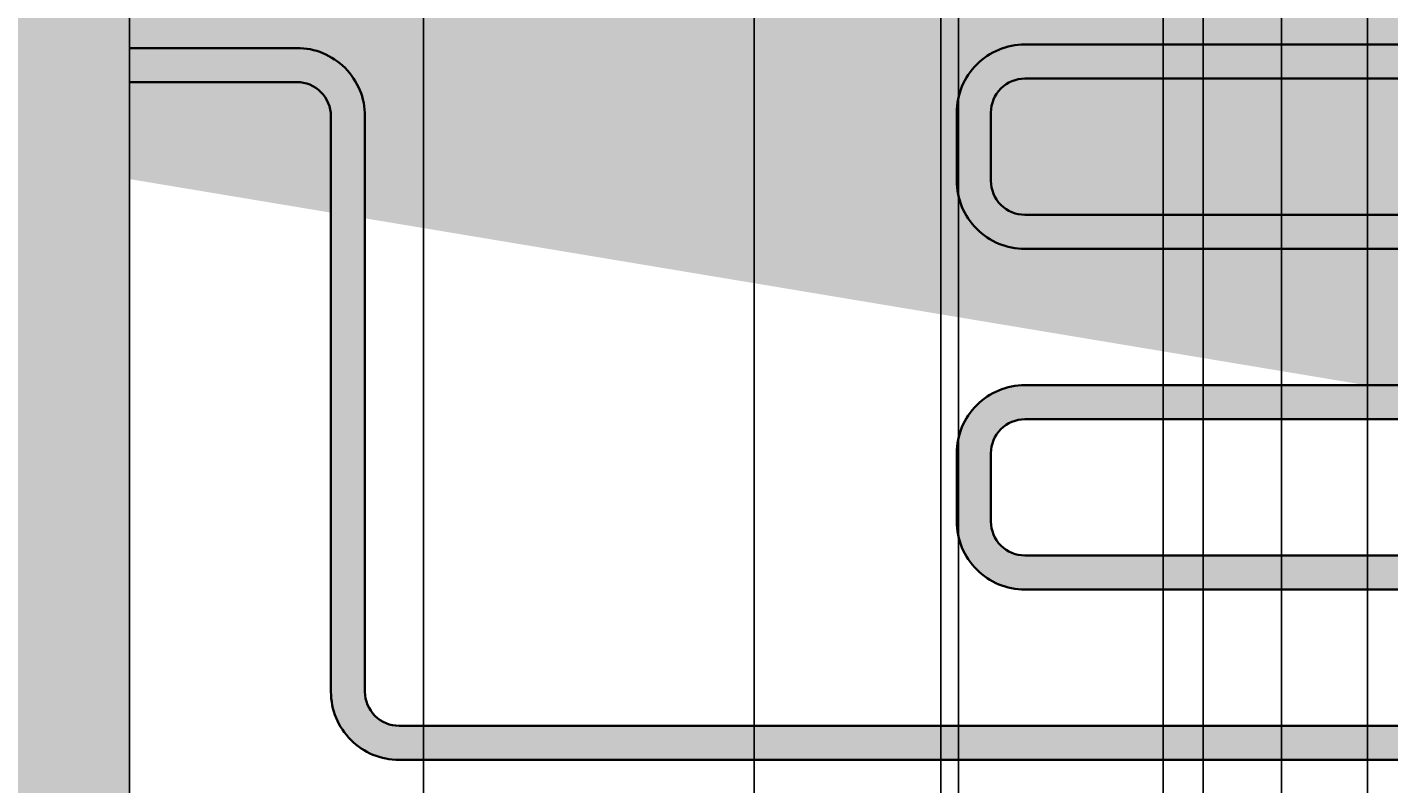
# Model space of a CAD drawing. Units: millimetres. Extents: x -22994 to 29398, y -19990 to 20176.
# Tile 32 of 135: x 99 to 139, y 56 to 78. Entities that reach past the tile are written whole.
import ezdxf

# ---------------------------------------------------------------- set-up
doc = ezdxf.new("R2010")
doc.units = ezdxf.units.MM
doc.header["$MEASUREMENT"] = 0
for name, color, linetype, lineweight in [('M-DIMS', 2, 'Continuous', 18), ('M-EQPM', 7, 'Continuous', 25), ('M-EQPM-PATT', 7, 'Continuous', 18), ('M-PIPE', 7, 'Continuous', 35)]:
    doc.layers.add(name, color=color, linetype=linetype, lineweight=lineweight)
doc.styles.get("Standard").update_dxf_attribs({"font": 'arial.ttf'})
doc.dimstyles.get("Standard").update_dxf_attribs({"dimtxt": 0.18, "dimasz": 10000, "dimexe": 0.18, "dimexo": 0.0625, "dimgap": 0.09, "dimtad": 0, "dimtih": 1, "dimtoh": 1, "dimdec": 0, "dimzin": 0, "dimdsep": 46, "dimtxsty": 'Standard', "dimcen": 0.09, "dimadec": 0, "dimazin": 0, "dimtfac": 1, "dimtdec": 0, "dimtofl": 0, "dimtmove": 0, "dimatfit": 3, "dimfxl": 1, "dimtolj": 1, "dimtzin": 0, "dimlwd": 30, "dimarcsym": 0})

# ---------------------------------------------------------------- blocks, each defined once
blk = doc.blocks.new('*D2')
at = {"layer": 'Defpoints', "color": 0, "transparency": 16777216}
for p in [(6.677, 10.271), (290.852, 10.271), (290.852, -5.079)]:
    blk.add_point(p, dxfattribs=at)
at = {"layer": 'M-DIMS', "color": 0, "lineweight": -2, "transparency": 16777216}
for p, q in [((6.677, 10.209), (6.677, -5.259)), ((290.852, 10.209), (290.852, -5.259))]:
    blk.add_line(p, q, dxfattribs=at)
at = {"layer": 'M-DIMS', "color": 0, "lineweight": 30, "transparency": 16777216}
for p, q in [((-9993.323, -5.079), (-19993.323, -5.079)), ((10290.852, -5.079), (20290.852, -5.079))]:
    blk.add_line(p, q, dxfattribs=at)
at = {"layer": 'M-DIMS', "color": 0, "transparency": 16777216}
for points in [[(-9993.323, 1661.588), (-9993.323, -1671.745), (6.677, -5.079)], [(10290.852, 1661.588), (10290.852, -1671.745), (290.852, -5.079)]]:
    blk.add_solid(points, dxfattribs=at)
at = {"layer": 'M-DIMS', "color": 0, "transparency": 16777216, "insert": (148.765, -5.079), "char_height": 0.18, "attachment_point": 5}
blk.add_mtext('\\A1;284.2', dxfattribs=at)
blk = doc.blocks.new('*D3')
at = {"layer": 'Defpoints', "color": 0, "transparency": 16777216}
for p in [(110.265, 204.165), (110.265, 176.366), (95.833, 127.967)]:
    blk.add_point(p, dxfattribs=at)
at = {"layer": 'M-DIMS', "color": 0, "lineweight": -2, "transparency": 16777216}
for p, q in [((95.833, 128.03), (95.833, 204.345)), ((110.265, 176.429), (110.265, 204.345))]:
    blk.add_line(p, q, dxfattribs=at)
at = {"layer": 'M-DIMS', "color": 0, "lineweight": 30, "transparency": 16777216}
for p, q in [((-9904.167, 204.165), (-19904.167, 204.165)), ((10110.265, 204.165), (20110.265, 204.165))]:
    blk.add_line(p, q, dxfattribs=at)
at = {"layer": 'M-DIMS', "color": 0, "transparency": 16777216}
for points in [[(-9904.167, 1870.832), (-9904.167, -1462.501), (95.833, 204.165)], [(10110.265, 1870.832), (10110.265, -1462.501), (110.265, 204.165)]]:
    blk.add_solid(points, dxfattribs=at)
at = {"layer": 'M-DIMS', "color": 0, "transparency": 16777216, "insert": (103.049, 204.165), "char_height": 0.18, "attachment_point": 5}
blk.add_mtext('\\A1;14.432', dxfattribs=at)
blk = doc.blocks.new('*D4')
at = {"layer": 'Defpoints', "color": 0, "transparency": 16777216}
for p in [(116.265, 204.165), (110.265, 176.366), (116.265, 176.366)]:
    blk.add_point(p, dxfattribs=at)
at = {"layer": 'M-DIMS', "color": 0, "lineweight": -2, "transparency": 16777216}
for p, q in [((110.265, 176.429), (110.265, 204.345)), ((116.265, 176.429), (116.265, 204.345))]:
    blk.add_line(p, q, dxfattribs=at)
at = {"layer": 'M-DIMS', "color": 0, "lineweight": 30, "transparency": 16777216}
for p, q in [((-9889.735, 204.165), (-19889.735, 204.165)), ((10116.265, 204.165), (20116.265, 204.165))]:
    blk.add_line(p, q, dxfattribs=at)
at = {"layer": 'M-DIMS', "color": 0, "transparency": 16777216}
for points in [[(-9889.735, 1870.832), (-9889.735, -1462.501), (110.265, 204.165)], [(10116.265, 1870.832), (10116.265, -1462.501), (116.265, 204.165)]]:
    blk.add_solid(points, dxfattribs=at)
at = {"layer": 'M-DIMS', "color": 0, "transparency": 16777216, "insert": (113.265, 204.165), "char_height": 0.18, "attachment_point": 5}
blk.add_mtext('\\A1;6', dxfattribs=at)
blk = doc.blocks.new('*D5')
at = {"layer": 'Defpoints', "color": 0, "transparency": 16777216}
for p in [(181.265, 204.165), (116.265, 176.366), (181.265, 176.366)]:
    blk.add_point(p, dxfattribs=at)
at = {"layer": 'M-DIMS', "color": 0, "lineweight": -2, "transparency": 16777216}
for p, q in [((116.265, 176.429), (116.265, 204.345)), ((181.265, 176.429), (181.265, 204.345))]:
    blk.add_line(p, q, dxfattribs=at)
at = {"layer": 'M-DIMS', "color": 0, "lineweight": 30, "transparency": 16777216}
for p, q in [((-9883.735, 204.165), (-19883.735, 204.165)), ((10181.265, 204.165), (20181.265, 204.165))]:
    blk.add_line(p, q, dxfattribs=at)
at = {"layer": 'M-DIMS', "color": 0, "transparency": 16777216}
for points in [[(-9883.735, 1870.832), (-9883.735, -1462.501), (116.265, 204.165)], [(10181.265, 1870.832), (10181.265, -1462.501), (181.265, 204.165)]]:
    blk.add_solid(points, dxfattribs=at)
at = {"layer": 'M-DIMS', "color": 0, "transparency": 16777216, "insert": (148.765, 204.165), "char_height": 0.18, "attachment_point": 5}
blk.add_mtext('\\A1;65', dxfattribs=at)
blk = doc.blocks.new('*D6')
at = {"layer": 'Defpoints', "color": 0, "transparency": 16777216}
for p in [(187.265, 204.165), (181.265, 176.366), (187.265, 176.366)]:
    blk.add_point(p, dxfattribs=at)
at = {"layer": 'M-DIMS', "color": 0, "lineweight": -2, "transparency": 16777216}
for p, q in [((181.265, 176.429), (181.265, 204.345)), ((187.265, 176.429), (187.265, 204.345))]:
    blk.add_line(p, q, dxfattribs=at)
at = {"layer": 'M-DIMS', "color": 0, "lineweight": 30, "transparency": 16777216}
for p, q in [((-9818.735, 204.165), (-19818.735, 204.165)), ((10187.265, 204.165), (20187.265, 204.165))]:
    blk.add_line(p, q, dxfattribs=at)
at = {"layer": 'M-DIMS', "color": 0, "transparency": 16777216}
for points in [[(-9818.735, 1870.832), (-9818.735, -1462.501), (181.265, 204.165)], [(10187.265, 1870.832), (10187.265, -1462.501), (187.265, 204.165)]]:
    blk.add_solid(points, dxfattribs=at)
at = {"layer": 'M-DIMS', "color": 0, "transparency": 16777216, "insert": (184.265, 204.165), "char_height": 0.18, "attachment_point": 5}
blk.add_mtext('\\A1;6', dxfattribs=at)
blk = doc.blocks.new('*D7')
at = {"layer": 'Defpoints', "color": 0, "transparency": 16777216}
for p in [(201.697, 204.165), (187.265, 176.366), (201.697, 127.967)]:
    blk.add_point(p, dxfattribs=at)
at = {"layer": 'M-DIMS', "color": 0, "lineweight": -2, "transparency": 16777216}
for p, q in [((187.265, 176.429), (187.265, 204.345)), ((201.697, 128.03), (201.697, 204.345))]:
    blk.add_line(p, q, dxfattribs=at)
at = {"layer": 'M-DIMS', "color": 0, "lineweight": 30, "transparency": 16777216}
for p, q in [((-9812.735, 204.165), (-19812.735, 204.165)), ((10201.697, 204.165), (20201.697, 204.165))]:
    blk.add_line(p, q, dxfattribs=at)
at = {"layer": 'M-DIMS', "color": 0, "transparency": 16777216}
for points in [[(-9812.735, 1870.832), (-9812.735, -1462.501), (187.265, 204.165)], [(10201.697, 1870.832), (10201.697, -1462.501), (201.697, 204.165)]]:
    blk.add_solid(points, dxfattribs=at)
at = {"layer": 'M-DIMS', "color": 0, "transparency": 16777216, "insert": (194.481, 204.165), "char_height": 0.18, "attachment_point": 5}
blk.add_mtext('\\A1;14.432', dxfattribs=at)
blk = doc.blocks.new('*D8')
at = {"layer": 'Defpoints', "color": 0, "transparency": 16777216}
for p in [(227.648, 204.165), (227.648, 146.73), (201.697, 127.967)]:
    blk.add_point(p, dxfattribs=at)
at = {"layer": 'M-DIMS', "color": 0, "lineweight": -2, "transparency": 16777216}
for p, q in [((201.697, 128.03), (201.697, 204.345)), ((227.648, 146.792), (227.648, 204.345))]:
    blk.add_line(p, q, dxfattribs=at)
at = {"layer": 'M-DIMS', "color": 0, "lineweight": 30, "transparency": 16777216}
for p, q in [((-9798.303, 204.165), (-19798.303, 204.165)), ((10227.648, 204.165), (20227.648, 204.165))]:
    blk.add_line(p, q, dxfattribs=at)
at = {"layer": 'M-DIMS', "color": 0, "transparency": 16777216}
for points in [[(-9798.303, 1870.832), (-9798.303, -1462.501), (201.697, 204.165)], [(10227.648, 1870.832), (10227.648, -1462.501), (227.648, 204.165)]]:
    blk.add_solid(points, dxfattribs=at)
at = {"layer": 'M-DIMS', "color": 0, "transparency": 16777216, "insert": (214.673, 204.165), "char_height": 0.18, "attachment_point": 5}
blk.add_mtext('\\A1;25.95', dxfattribs=at)
blk = doc.blocks.new('*D9')
at = {"layer": 'Defpoints', "color": 0, "transparency": 16777216}
for p in [(187.265, 176.366), (306.202, 176.366), (290.852, 10.271)]:
    blk.add_point(p, dxfattribs=at)
at = {"layer": 'M-DIMS', "color": 0, "lineweight": 30, "transparency": 16777216}
for p, q in [((306.202, 10176.366), (306.202, 20176.366)), ((306.202, -9989.729), (306.202, -19989.729))]:
    blk.add_line(p, q, dxfattribs=at)
at = {"layer": 'M-DIMS', "color": 0, "lineweight": -2, "transparency": 16777216}
for p, q in [((187.327, 176.366), (306.382, 176.366)), ((290.915, 10.271), (306.382, 10.271))]:
    blk.add_line(p, q, dxfattribs=at)
at = {"layer": 'M-DIMS', "color": 0, "transparency": 16777216}
for points in [[(-1360.465, 10176.366), (1972.869, 10176.366), (306.202, 176.366)], [(-1360.465, -9989.729), (1972.869, -9989.729), (306.202, 10.271)]]:
    blk.add_solid(points, dxfattribs=at)
at = {"layer": 'M-DIMS', "color": 0, "transparency": 16777216, "insert": (306.202, 93.319), "char_height": 0.18, "attachment_point": 5}
blk.add_mtext('\\A1;166.1', dxfattribs=at)
blk = doc.blocks.new('*D10')
at = {"layer": 'Defpoints', "color": 0, "transparency": 16777216}
for p in [(125.65, 136.071), (133.346, 136.071), (133.346, -5.079)]:
    blk.add_point(p, dxfattribs=at)
at = {"layer": 'M-DIMS', "color": 0, "lineweight": -2, "transparency": 16777216}
for p, q in [((125.65, 136.009), (125.65, -5.259)), ((133.346, 136.009), (133.346, -5.259))]:
    blk.add_line(p, q, dxfattribs=at)
at = {"layer": 'M-DIMS', "color": 0, "lineweight": 30, "transparency": 16777216}
for p, q in [((-9874.35, -5.079), (-19874.35, -5.079)), ((10133.346, -5.079), (20133.346, -5.079))]:
    blk.add_line(p, q, dxfattribs=at)
at = {"layer": 'M-DIMS', "color": 0, "transparency": 16777216}
for points in [[(-9874.35, 1661.588), (-9874.35, -1671.745), (125.65, -5.079)], [(10133.346, 1661.588), (10133.346, -1671.745), (133.346, -5.079)]]:
    blk.add_solid(points, dxfattribs=at)
at = {"layer": 'M-DIMS', "color": 0, "transparency": 16777216, "insert": (129.498, -5.079), "char_height": 0.18, "attachment_point": 5}
blk.add_mtext('\\A1;7.696', dxfattribs=at)
blk = doc.blocks.new('*D11')
at = {"layer": 'Defpoints', "color": 0, "transparency": 16777216}
for p in [(133.346, 136.071), (135.65, 136.071), (135.65, -5.079)]:
    blk.add_point(p, dxfattribs=at)
at = {"layer": 'M-DIMS', "color": 0, "lineweight": -2, "transparency": 16777216}
for p, q in [((133.346, 136.009), (133.346, -5.259)), ((135.65, 136.009), (135.65, -5.259))]:
    blk.add_line(p, q, dxfattribs=at)
at = {"layer": 'M-DIMS', "color": 0, "lineweight": 30, "transparency": 16777216}
for p, q in [((-9866.654, -5.079), (-19866.654, -5.079)), ((10135.65, -5.079), (20135.65, -5.079))]:
    blk.add_line(p, q, dxfattribs=at)
at = {"layer": 'M-DIMS', "color": 0, "transparency": 16777216}
for points in [[(-9866.654, 1661.588), (-9866.654, -1671.745), (133.346, -5.079)], [(10135.65, 1661.588), (10135.65, -1671.745), (135.65, -5.079)]]:
    blk.add_solid(points, dxfattribs=at)
at = {"layer": 'M-DIMS', "color": 0, "transparency": 16777216, "insert": (134.498, -5.079), "char_height": 0.18, "attachment_point": 5}
blk.add_mtext('\\A1;2.304', dxfattribs=at)
blk = doc.blocks.new('*D12')
at = {"layer": 'Defpoints', "color": 0, "transparency": 16777216}
for p in [(135.65, 136.071), (145.65, 136.071), (145.65, -5.079)]:
    blk.add_point(p, dxfattribs=at)
at = {"layer": 'M-DIMS', "color": 0, "lineweight": -2, "transparency": 16777216}
for p, q in [((135.65, 136.009), (135.65, -5.259)), ((145.65, 136.009), (145.65, -5.259))]:
    blk.add_line(p, q, dxfattribs=at)
at = {"layer": 'M-DIMS', "color": 0, "lineweight": 30, "transparency": 16777216}
for p, q in [((-9864.35, -5.079), (-19864.35, -5.079)), ((10145.65, -5.079), (20145.65, -5.079))]:
    blk.add_line(p, q, dxfattribs=at)
at = {"layer": 'M-DIMS', "color": 0, "transparency": 16777216}
for points in [[(-9864.35, 1661.588), (-9864.35, -1671.745), (135.65, -5.079)], [(10145.65, 1661.588), (10145.65, -1671.745), (145.65, -5.079)]]:
    blk.add_solid(points, dxfattribs=at)
at = {"layer": 'M-DIMS', "color": 0, "transparency": 16777216, "insert": (140.65, -5.079), "char_height": 0.18, "attachment_point": 5}
blk.add_mtext('\\A1;10', dxfattribs=at)
blk = doc.blocks.new('*D13')
at = {"layer": 'Defpoints', "color": 0, "transparency": 16777216}
for p in [(145.65, 136.071), (155.65, 136.071), (155.65, -5.079)]:
    blk.add_point(p, dxfattribs=at)
at = {"layer": 'M-DIMS', "color": 0, "lineweight": -2, "transparency": 16777216}
for p, q in [((145.65, 136.009), (145.65, -5.259)), ((155.65, 136.009), (155.65, -5.259))]:
    blk.add_line(p, q, dxfattribs=at)
at = {"layer": 'M-DIMS', "color": 0, "lineweight": 30, "transparency": 16777216}
for p, q in [((-9854.35, -5.079), (-19854.35, -5.079)), ((10155.65, -5.079), (20155.65, -5.079))]:
    blk.add_line(p, q, dxfattribs=at)
at = {"layer": 'M-DIMS', "color": 0, "transparency": 16777216}
for points in [[(-9854.35, 1661.588), (-9854.35, -1671.745), (145.65, -5.079)], [(10155.65, 1661.588), (10155.65, -1671.745), (155.65, -5.079)]]:
    blk.add_solid(points, dxfattribs=at)
at = {"layer": 'M-DIMS', "color": 0, "transparency": 16777216, "insert": (150.65, -5.079), "char_height": 0.18, "attachment_point": 5}
blk.add_mtext('\\A1;10', dxfattribs=at)
blk = doc.blocks.new('*D14')
at = {"layer": 'Defpoints', "color": 0, "transparency": 16777216}
for p in [(155.65, 136.071), (165.65, 136.071), (165.65, -5.079)]:
    blk.add_point(p, dxfattribs=at)
at = {"layer": 'M-DIMS', "color": 0, "lineweight": -2, "transparency": 16777216}
for p, q in [((155.65, 136.009), (155.65, -5.259)), ((165.65, 136.009), (165.65, -5.259))]:
    blk.add_line(p, q, dxfattribs=at)
at = {"layer": 'M-DIMS', "color": 0, "lineweight": 30, "transparency": 16777216}
for p, q in [((-9844.35, -5.079), (-19844.35, -5.079)), ((10165.65, -5.079), (20165.65, -5.079))]:
    blk.add_line(p, q, dxfattribs=at)
at = {"layer": 'M-DIMS', "color": 0, "transparency": 16777216}
for points in [[(-9844.35, 1661.588), (-9844.35, -1671.745), (155.65, -5.079)], [(10165.65, 1661.588), (10165.65, -1671.745), (165.65, -5.079)]]:
    blk.add_solid(points, dxfattribs=at)
at = {"layer": 'M-DIMS', "color": 0, "transparency": 16777216, "insert": (160.65, -5.079), "char_height": 0.18, "attachment_point": 5}
blk.add_mtext('\\A1;10', dxfattribs=at)
blk = doc.blocks.new('*D15')
at = {"layer": 'Defpoints', "color": 0, "transparency": 16777216}
for p in [(173.346, 154.788), (173.346, 136.071), (306.202, 136.071)]:
    blk.add_point(p, dxfattribs=at)
at = {"layer": 'M-DIMS', "color": 0, "lineweight": 30, "transparency": 16777216}
for p, q in [((306.202, 10154.788), (306.202, 20154.788)), ((306.202, -9863.929), (306.202, -19863.929))]:
    blk.add_line(p, q, dxfattribs=at)
at = {"layer": 'M-DIMS', "color": 0, "lineweight": -2, "transparency": 16777216}
for p, q in [((173.408, 154.788), (306.382, 154.788)), ((173.408, 136.071), (306.382, 136.071))]:
    blk.add_line(p, q, dxfattribs=at)
at = {"layer": 'M-DIMS', "color": 0, "transparency": 16777216}
for points in [[(-1360.465, 10154.788), (1972.869, 10154.788), (306.202, 154.788)], [(-1360.465, -9863.929), (1972.869, -9863.929), (306.202, 136.071)]]:
    blk.add_solid(points, dxfattribs=at)
at = {"layer": 'M-DIMS', "color": 0, "transparency": 16777216, "insert": (306.202, 145.43), "char_height": 0.18, "attachment_point": 5}
blk.add_mtext('\\A1;18.717', dxfattribs=at)
blk = doc.blocks.new('*D16')
at = {"layer": 'Defpoints', "color": 0, "transparency": 16777216}
for p in [(120.17, 204.165), (110.466, 48.035), (120.17, 48.035)]:
    blk.add_point(p, dxfattribs=at)
at = {"layer": 'M-DIMS', "color": 0, "lineweight": -2, "transparency": 16777216}
for p, q in [((110.466, 48.097), (110.466, 204.345)), ((120.17, 48.097), (120.17, 204.345))]:
    blk.add_line(p, q, dxfattribs=at)
at = {"layer": 'M-DIMS', "color": 0, "lineweight": 30, "transparency": 16777216}
for p, q in [((-9889.534, 204.165), (-19889.534, 204.165)), ((10120.17, 204.165), (20120.17, 204.165))]:
    blk.add_line(p, q, dxfattribs=at)
at = {"layer": 'M-DIMS', "color": 0, "transparency": 16777216}
for points in [[(-9889.534, 1870.832), (-9889.534, -1462.501), (110.466, 204.165)], [(10120.17, 1870.832), (10120.17, -1462.501), (120.17, 204.165)]]:
    blk.add_solid(points, dxfattribs=at)
at = {"layer": 'M-DIMS', "color": 0, "transparency": 16777216, "insert": (115.318, 204.165), "char_height": 0.18, "attachment_point": 5}
blk.add_mtext('\\A1;9.704', dxfattribs=at)
blk = doc.blocks.new('*D17')
at = {"layer": 'Defpoints', "color": 0, "transparency": 16777216}
for p in [(126.17, 204.165), (120.17, 48.035), (126.17, 48.035)]:
    blk.add_point(p, dxfattribs=at)
at = {"layer": 'M-DIMS', "color": 0, "lineweight": -2, "transparency": 16777216}
for p, q in [((120.17, 48.097), (120.17, 204.345)), ((126.17, 48.097), (126.17, 204.345))]:
    blk.add_line(p, q, dxfattribs=at)
at = {"layer": 'M-DIMS', "color": 0, "lineweight": 30, "transparency": 16777216}
for p, q in [((-9879.83, 204.165), (-19879.83, 204.165)), ((10126.17, 204.165), (20126.17, 204.165))]:
    blk.add_line(p, q, dxfattribs=at)
at = {"layer": 'M-DIMS', "color": 0, "transparency": 16777216}
for points in [[(-9879.83, 1870.832), (-9879.83, -1462.501), (120.17, 204.165)], [(10126.17, 1870.832), (10126.17, -1462.501), (126.17, 204.165)]]:
    blk.add_solid(points, dxfattribs=at)
at = {"layer": 'M-DIMS', "color": 0, "transparency": 16777216, "insert": (123.17, 204.165), "char_height": 0.18, "attachment_point": 5}
blk.add_mtext('\\A1;6', dxfattribs=at)
blk = doc.blocks.new('*D18')
at = {"layer": 'Defpoints', "color": 0, "transparency": 16777216}
for p in [(132.17, 204.165), (126.17, 48.035), (132.17, 48.035)]:
    blk.add_point(p, dxfattribs=at)
at = {"layer": 'M-DIMS', "color": 0, "lineweight": -2, "transparency": 16777216}
for p, q in [((126.17, 48.097), (126.17, 204.345)), ((132.17, 48.097), (132.17, 204.345))]:
    blk.add_line(p, q, dxfattribs=at)
at = {"layer": 'M-DIMS', "color": 0, "lineweight": 30, "transparency": 16777216}
for p, q in [((-9873.83, 204.165), (-19873.83, 204.165)), ((10132.17, 204.165), (20132.17, 204.165))]:
    blk.add_line(p, q, dxfattribs=at)
at = {"layer": 'M-DIMS', "color": 0, "transparency": 16777216}
for points in [[(-9873.83, 1870.832), (-9873.83, -1462.501), (126.17, 204.165)], [(10132.17, 1870.832), (10132.17, -1462.501), (132.17, 204.165)]]:
    blk.add_solid(points, dxfattribs=at)
at = {"layer": 'M-DIMS', "color": 0, "transparency": 16777216, "insert": (129.17, 204.165), "char_height": 0.18, "attachment_point": 5}
blk.add_mtext('\\A1;6', dxfattribs=at)
blk = doc.blocks.new('*D19')
at = {"layer": 'Defpoints', "color": 0, "transparency": 16777216}
for p in [(138.17, 204.165), (132.17, 48.035), (138.17, 48.035)]:
    blk.add_point(p, dxfattribs=at)
at = {"layer": 'M-DIMS', "color": 0, "lineweight": -2, "transparency": 16777216}
for p, q in [((132.17, 48.097), (132.17, 204.345)), ((138.17, 48.097), (138.17, 204.345))]:
    blk.add_line(p, q, dxfattribs=at)
at = {"layer": 'M-DIMS', "color": 0, "lineweight": 30, "transparency": 16777216}
for p, q in [((-9867.83, 204.165), (-19867.83, 204.165)), ((10138.17, 204.165), (20138.17, 204.165))]:
    blk.add_line(p, q, dxfattribs=at)
at = {"layer": 'M-DIMS', "color": 0, "transparency": 16777216}
for points in [[(-9867.83, 1870.832), (-9867.83, -1462.501), (132.17, 204.165)], [(10138.17, 1870.832), (10138.17, -1462.501), (138.17, 204.165)]]:
    blk.add_solid(points, dxfattribs=at)
at = {"layer": 'M-DIMS', "color": 0, "transparency": 16777216, "insert": (135.17, 204.165), "char_height": 0.18, "attachment_point": 5}
blk.add_mtext('\\A1;6', dxfattribs=at)
blk = doc.blocks.new('*D20')
at = {"layer": 'Defpoints', "color": 0, "transparency": 16777216}
for p in [(144.17, 204.165), (138.17, 48.035), (144.17, 48.035)]:
    blk.add_point(p, dxfattribs=at)
at = {"layer": 'M-DIMS', "color": 0, "lineweight": -2, "transparency": 16777216}
for p, q in [((138.17, 48.097), (138.17, 204.345)), ((144.17, 48.097), (144.17, 204.345))]:
    blk.add_line(p, q, dxfattribs=at)
at = {"layer": 'M-DIMS', "color": 0, "lineweight": 30, "transparency": 16777216}
for p, q in [((-9861.83, 204.165), (-19861.83, 204.165)), ((10144.17, 204.165), (20144.17, 204.165))]:
    blk.add_line(p, q, dxfattribs=at)
at = {"layer": 'M-DIMS', "color": 0, "transparency": 16777216}
for points in [[(-9861.83, 1870.832), (-9861.83, -1462.501), (138.17, 204.165)], [(10144.17, 1870.832), (10144.17, -1462.501), (144.17, 204.165)]]:
    blk.add_solid(points, dxfattribs=at)
at = {"layer": 'M-DIMS', "color": 0, "transparency": 16777216, "insert": (141.17, 204.165), "char_height": 0.18, "attachment_point": 5}
blk.add_mtext('\\A1;6', dxfattribs=at)
blk = doc.blocks.new('*D21')
at = {"layer": 'Defpoints', "color": 0, "transparency": 16777216}
for p in [(149.116, 204.165), (144.17, 48.035), (149.116, 48.035)]:
    blk.add_point(p, dxfattribs=at)
at = {"layer": 'M-DIMS', "color": 0, "lineweight": -2, "transparency": 16777216}
for p, q in [((144.17, 48.097), (144.17, 204.345)), ((149.116, 48.097), (149.116, 204.345))]:
    blk.add_line(p, q, dxfattribs=at)
at = {"layer": 'M-DIMS', "color": 0, "lineweight": 30, "transparency": 16777216}
for p, q in [((-9855.83, 204.165), (-19855.83, 204.165)), ((10149.116, 204.165), (20149.116, 204.165))]:
    blk.add_line(p, q, dxfattribs=at)
at = {"layer": 'M-DIMS', "color": 0, "transparency": 16777216}
for points in [[(-9855.83, 1870.832), (-9855.83, -1462.501), (144.17, 204.165)], [(10149.116, 1870.832), (10149.116, -1462.501), (149.116, 204.165)]]:
    blk.add_solid(points, dxfattribs=at)
at = {"layer": 'M-DIMS', "color": 0, "transparency": 16777216, "insert": (146.643, 204.165), "char_height": 0.18, "attachment_point": 5}
blk.add_mtext('\\A1;4.945', dxfattribs=at)
blk = doc.blocks.new('*D22')
at = {"layer": 'Defpoints', "color": 0, "transparency": 16777216}
for p in [(149.116, 30.99), (155.116, 30.99), (155.116, -5.079)]:
    blk.add_point(p, dxfattribs=at)
at = {"layer": 'M-DIMS', "color": 0, "lineweight": -2, "transparency": 16777216}
for p, q in [((149.116, 30.927), (149.116, -5.259)), ((155.116, 30.927), (155.116, -5.259))]:
    blk.add_line(p, q, dxfattribs=at)
at = {"layer": 'M-DIMS', "color": 0, "lineweight": 30, "transparency": 16777216}
for p, q in [((-9850.884, -5.079), (-19850.884, -5.079)), ((10155.116, -5.079), (20155.116, -5.079))]:
    blk.add_line(p, q, dxfattribs=at)
at = {"layer": 'M-DIMS', "color": 0, "transparency": 16777216}
for points in [[(-9850.884, 1661.588), (-9850.884, -1671.745), (149.116, -5.079)], [(10155.116, 1661.588), (10155.116, -1671.745), (155.116, -5.079)]]:
    blk.add_solid(points, dxfattribs=at)
at = {"layer": 'M-DIMS', "color": 0, "transparency": 16777216, "insert": (152.116, -5.079), "char_height": 0.18, "attachment_point": 5}
blk.add_mtext('\\A1;6', dxfattribs=at)
blk = doc.blocks.new('*D23')
at = {"layer": 'Defpoints', "color": 0, "transparency": 16777216}
for p in [(155.116, 30.99), (161.116, 30.99), (161.116, -5.079)]:
    blk.add_point(p, dxfattribs=at)
at = {"layer": 'M-DIMS', "color": 0, "lineweight": -2, "transparency": 16777216}
for p, q in [((155.116, 30.927), (155.116, -5.259)), ((161.116, 30.927), (161.116, -5.259))]:
    blk.add_line(p, q, dxfattribs=at)
at = {"layer": 'M-DIMS', "color": 0, "lineweight": 30, "transparency": 16777216}
for p, q in [((-9844.884, -5.079), (-19844.884, -5.079)), ((10161.116, -5.079), (20161.116, -5.079))]:
    blk.add_line(p, q, dxfattribs=at)
at = {"layer": 'M-DIMS', "color": 0, "transparency": 16777216}
for points in [[(-9844.884, 1661.588), (-9844.884, -1671.745), (155.116, -5.079)], [(10161.116, 1661.588), (10161.116, -1671.745), (161.116, -5.079)]]:
    blk.add_solid(points, dxfattribs=at)
at = {"layer": 'M-DIMS', "color": 0, "transparency": 16777216, "insert": (158.116, -5.079), "char_height": 0.18, "attachment_point": 5}
blk.add_mtext('\\A1;6', dxfattribs=at)
blk = doc.blocks.new('*D24')
at = {"layer": 'Defpoints', "color": 0, "transparency": 16777216}
for p in [(161.116, 30.99), (166.439, 30.99), (166.439, -5.079)]:
    blk.add_point(p, dxfattribs=at)
at = {"layer": 'M-DIMS', "color": 0, "lineweight": -2, "transparency": 16777216}
for p, q in [((161.116, 30.927), (161.116, -5.259)), ((166.439, 30.927), (166.439, -5.259))]:
    blk.add_line(p, q, dxfattribs=at)
at = {"layer": 'M-DIMS', "color": 0, "lineweight": 30, "transparency": 16777216}
for p, q in [((-9838.884, -5.079), (-19838.884, -5.079)), ((10166.439, -5.079), (20166.439, -5.079))]:
    blk.add_line(p, q, dxfattribs=at)
at = {"layer": 'M-DIMS', "color": 0, "transparency": 16777216}
for points in [[(-9838.884, 1661.588), (-9838.884, -1671.745), (161.116, -5.079)], [(10166.439, 1661.588), (10166.439, -1671.745), (166.439, -5.079)]]:
    blk.add_solid(points, dxfattribs=at)
at = {"layer": 'M-DIMS', "color": 0, "transparency": 16777216, "insert": (163.777, -5.079), "char_height": 0.18, "attachment_point": 5}
blk.add_mtext('\\A1;5.323', dxfattribs=at)
blk = doc.blocks.new('*D25')
at = {"layer": 'Defpoints', "color": 0, "transparency": 16777216}
for p in [(166.439, 30.99), (172.439, 30.99), (172.439, -5.079)]:
    blk.add_point(p, dxfattribs=at)
at = {"layer": 'M-DIMS', "color": 0, "lineweight": -2, "transparency": 16777216}
for p, q in [((166.439, 30.927), (166.439, -5.259)), ((172.439, 30.927), (172.439, -5.259))]:
    blk.add_line(p, q, dxfattribs=at)
at = {"layer": 'M-DIMS', "color": 0, "lineweight": 30, "transparency": 16777216}
for p, q in [((-9833.561, -5.079), (-19833.561, -5.079)), ((10172.439, -5.079), (20172.439, -5.079))]:
    blk.add_line(p, q, dxfattribs=at)
at = {"layer": 'M-DIMS', "color": 0, "transparency": 16777216}
for points in [[(-9833.561, 1661.588), (-9833.561, -1671.745), (166.439, -5.079)], [(10172.439, 1661.588), (10172.439, -1671.745), (172.439, -5.079)]]:
    blk.add_solid(points, dxfattribs=at)
at = {"layer": 'M-DIMS', "color": 0, "transparency": 16777216, "insert": (169.439, -5.079), "char_height": 0.18, "attachment_point": 5}
blk.add_mtext('\\A1;6', dxfattribs=at)
blk = doc.blocks.new('*D26')
at = {"layer": 'Defpoints', "color": 0, "transparency": 16777216}
for p in [(172.439, 30.99), (178.439, 30.99), (178.439, -5.079)]:
    blk.add_point(p, dxfattribs=at)
at = {"layer": 'M-DIMS', "color": 0, "lineweight": -2, "transparency": 16777216}
for p, q in [((172.439, 30.927), (172.439, -5.259)), ((178.439, 30.927), (178.439, -5.259))]:
    blk.add_line(p, q, dxfattribs=at)
at = {"layer": 'M-DIMS', "color": 0, "lineweight": 30, "transparency": 16777216}
for p, q in [((-9827.561, -5.079), (-19827.561, -5.079)), ((10178.439, -5.079), (20178.439, -5.079))]:
    blk.add_line(p, q, dxfattribs=at)
at = {"layer": 'M-DIMS', "color": 0, "transparency": 16777216}
for points in [[(-9827.561, 1661.588), (-9827.561, -1671.745), (172.439, -5.079)], [(10178.439, 1661.588), (10178.439, -1671.745), (178.439, -5.079)]]:
    blk.add_solid(points, dxfattribs=at)
at = {"layer": 'M-DIMS', "color": 0, "transparency": 16777216, "insert": (175.439, -5.079), "char_height": 0.18, "attachment_point": 5}
blk.add_mtext('\\A1;6', dxfattribs=at)
blk = doc.blocks.new('*D27')
at = {"layer": 'Defpoints', "color": 0, "transparency": 16777216}
for p in [(178.439, 30.99), (188.117, 30.99), (188.117, -5.079)]:
    blk.add_point(p, dxfattribs=at)
at = {"layer": 'M-DIMS', "color": 0, "lineweight": -2, "transparency": 16777216}
for p, q in [((178.439, 30.927), (178.439, -5.259)), ((188.117, 30.927), (188.117, -5.259))]:
    blk.add_line(p, q, dxfattribs=at)
at = {"layer": 'M-DIMS', "color": 0, "lineweight": 30, "transparency": 16777216}
for p, q in [((-9821.561, -5.079), (-19821.561, -5.079)), ((10188.117, -5.079), (20188.117, -5.079))]:
    blk.add_line(p, q, dxfattribs=at)
at = {"layer": 'M-DIMS', "color": 0, "transparency": 16777216}
for points in [[(-9821.561, 1661.588), (-9821.561, -1671.745), (178.439, -5.079)], [(10188.117, 1661.588), (10188.117, -1671.745), (188.117, -5.079)]]:
    blk.add_solid(points, dxfattribs=at)
at = {"layer": 'M-DIMS', "color": 0, "transparency": 16777216, "insert": (183.278, -5.079), "char_height": 0.18, "attachment_point": 5}
blk.add_mtext('\\A1;9.679', dxfattribs=at)
blk = doc.blocks.new('*D28')
at = {"layer": 'Defpoints', "color": 0, "transparency": 16777216}
for p in [(188.117, 48.035), (306.202, 48.035), (188.117, 30.99)]:
    blk.add_point(p, dxfattribs=at)
at = {"layer": 'M-DIMS', "color": 0, "lineweight": 30, "transparency": 16777216}
for p, q in [((306.202, 10048.035), (306.202, 20048.035)), ((306.202, -9969.01), (306.202, -19969.01))]:
    blk.add_line(p, q, dxfattribs=at)
at = {"layer": 'M-DIMS', "color": 0, "lineweight": -2, "transparency": 16777216}
for p, q in [((188.18, 48.035), (306.382, 48.035)), ((188.18, 30.99), (306.382, 30.99))]:
    blk.add_line(p, q, dxfattribs=at)
at = {"layer": 'M-DIMS', "color": 0, "transparency": 16777216}
for points in [[(-1360.465, 10048.035), (1972.869, 10048.035), (306.202, 48.035)], [(-1360.465, -9969.01), (1972.869, -9969.01), (306.202, 30.99)]]:
    blk.add_solid(points, dxfattribs=at)
at = {"layer": 'M-DIMS', "color": 0, "transparency": 16777216, "insert": (306.202, 39.512), "char_height": 0.18, "attachment_point": 5}
blk.add_mtext('\\A1;17.045', dxfattribs=at)
blk = doc.blocks.new('*D29')
at = {"layer": 'Defpoints', "color": 0, "transparency": 16777216}
for p in [(36.801, 80.045), (64.03, 80.045)]:
    blk.add_point(p, dxfattribs=at)
at = {"layer": 'M-DIMS', "color": 0, "lineweight": -2, "transparency": 16777216}
for p, q in [((50.325, 80.045), (50.505, 80.045)), ((50.415, 79.955), (50.415, 80.135))]:
    blk.add_line(p, q, dxfattribs=at)
at = {"layer": 'M-DIMS', "color": 0, "lineweight": 30, "transparency": 16777216}
blk.add_line((20064.03, 80.03), (10064.03, 80.038), dxfattribs=at)
at = {"layer": 'M-DIMS', "color": 0, "transparency": 16777216}
blk.add_solid([(10064.031, 1746.704), (10064.028, -1586.629), (64.03, 80.045)], dxfattribs=at)
at = {"layer": 'M-DIMS', "color": 0, "transparency": 16777216, "insert": (20064.521, 80.03), "char_height": 0.18, "attachment_point": 5}
blk.add_mtext('\\A1;∅27.23', dxfattribs=at)
blk = doc.blocks.new('*D36')
at = {"layer": 'Defpoints', "color": 0, "transparency": 16777216}
for p in [(46.39, 31.303), (46.387, 26.593)]:
    blk.add_point(p, dxfattribs=at)
at = {"layer": 'M-DIMS', "color": 0, "lineweight": 30, "transparency": 16777216}
for p, q in [((57.15, 20031.301), (51.77, 10031.302)), ((10057.15, 20031.301), (57.15, 20031.301))]:
    blk.add_line(p, q, dxfattribs=at)
at = {"layer": 'M-DIMS', "color": 0, "lineweight": -2, "transparency": 16777216}
for p, q in [((46.299, 28.948), (46.479, 28.948)), ((46.389, 28.858), (46.389, 29.038))]:
    blk.add_line(p, q, dxfattribs=at)
at = {"layer": 'M-DIMS', "color": 0, "transparency": 16777216}
blk.add_solid([(-1614.896, 10032.199), (1718.436, 10030.405), (46.39, 31.303)], dxfattribs=at)
at = {"layer": 'M-DIMS', "color": 0, "transparency": 16777216, "insert": (10057.554, 20031.301), "char_height": 0.18, "attachment_point": 5}
blk.add_mtext('\\A1;∅4.71', dxfattribs=at)
blk = doc.blocks.new('*D37')
at = {"layer": 'Defpoints', "color": 0, "transparency": 16777216}
for p in [(54.834, 118.615), (59.494, 118.614)]:
    blk.add_point(p, dxfattribs=at)
at = {"layer": 'M-DIMS', "color": 0, "lineweight": -2, "transparency": 16777216}
for p, q in [((57.164, 118.524), (57.164, 118.704)), ((57.074, 118.614), (57.254, 118.614))]:
    blk.add_line(p, q, dxfattribs=at)
at = {"layer": 'M-DIMS', "color": 0, "lineweight": 30, "transparency": 16777216}
blk.add_line((20059.493, 116.253), (10059.494, 117.434), dxfattribs=at)
at = {"layer": 'M-DIMS', "color": 0, "transparency": 16777216}
blk.add_solid([(10059.69, 1784.1), (10059.297, -1549.233), (59.494, 118.614)], dxfattribs=at)
at = {"layer": 'M-DIMS', "color": 0, "transparency": 16777216, "insert": (20059.985, 116.253), "char_height": 0.18, "attachment_point": 5}
blk.add_mtext('\\A1;∅4.659', dxfattribs=at)

msp = doc.modelspace()

# ---------------------------------------------------------------- hatches: boundary and pattern name
at = {"layer": 'M-EQPM-PATT'}
h = msp.add_hatch(color=256, dxfattribs=at)
h.set_gradient(color1=(205, 32, 39), color2=(205, 32, 39), tint=1)
h.paths.add_polyline_path([(116.2647, 150.3662), (116.2647, 170.3662), (116.2647, 176.3662), (110.2647, 176.3662), (110.2647, 152.0276), (95.8327, 127.967), (95.8327, 16.6063), (201.6967, 16.6063), (201.6967, 127.967), (187.2647, 152.0276), (187.2647, 176.3662), (181.2647, 176.3662), (181.2647, 170.3662), (181.2647, 150.3662), (195.6967, 126.3055), (195.6967, 22.6063), (101.8327, 22.6063), (101.8327, 126.3055)])
h.paths.add_polyline_path([(185.2208, 88.6347), (101.8327, 88.6347), (101.8327, 87.6347), (182.8066, 87.6347), (178.7313, 83.5594), (195.6967, 83.5594), (195.6967, 84.5594), (181.1455, 84.5594)], flags=17)
h.paths.add_polyline_path([(95.8327, 88.6347), (60.9779, 88.6347, -0.0228552), (61.7178, 87.6347), (95.8327, 87.6347)])
h.paths.add_polyline_path([(215.6212, 86.5189), (215.6212, 80.5999), (220.5095, 83.5594)])
h.paths.add_polyline_path([(215.6212, 84.5594), (201.6967, 84.5594), (201.6967, 83.5594), (215.6212, 83.5594)])
h.paths.add_polyline_path([(225.3978, 86.5189), (220.5095, 83.5594), (225.3978, 80.5999)])
h.paths.add_polyline_path([(231.6256, 84.5594), (225.3978, 84.5594), (225.3978, 83.5594), (231.6256, 83.5594)])
h = msp.add_hatch(color=256, dxfattribs=at)
h.set_gradient(color1=(19, 155, 72), color2=(88, 186, 72), tint=1, name='CYLINDER')
h.paths.add_polyline_path([(109.4658, 29.9895), (189.1175, 29.9895), (189.1175, 77.6953), (128.1172, 77.6953, 0.4142136), (126.1172, 75.6953), (126.1172, 73.6953, 0.4142136), (128.1172, 71.6953), (178.5136, 71.6953, -0.4142136), (179.5136, 70.6953), (179.5136, 68.6953, -0.4142136), (178.5136, 67.6953), (128.1172, 67.6953, 0.4142136), (126.1172, 65.6953), (126.1172, 63.6953, 0.4142136), (128.1172, 61.6953), (178.5136, 61.6953, -0.4142136), (179.5136, 60.6953), (179.5136, 58.6953, -0.4142136), (178.5136, 57.6953), (109.7466, 57.6953, -0.4142136), (108.7466, 58.6953), (108.7466, 75.5922, 0.4142136), (106.7466, 77.5922), (101.8327, 77.5922), (101.8327, 76.5922), (106.7466, 76.5922, -0.4142136), (107.7466, 75.5922), (107.7466, 58.6953, 0.4142136), (109.7466, 56.6953), (178.5136, 56.6953, 0.4142136), (180.5136, 58.6953), (180.5136, 60.6953, 0.4142136), (178.5136, 62.6953), (128.1172, 62.6953, -0.4142136), (127.1172, 63.6953), (127.1172, 65.6953, -0.4142136), (128.1172, 66.6953), (178.5136, 66.6953, 0.4142136), (180.5136, 68.6953), (180.5136, 70.6953, 0.4142136), (178.5136, 72.6953), (128.1172, 72.6953, -0.4142136), (127.1172, 73.6953), (127.1172, 75.6953, -0.4142136), (128.1172, 76.6953), (188.1175, 76.6953), (188.1175, 49.0349), (110.4658, 49.0349), (110.4658, 51.9576), (101.8327, 51.9576), (101.8327, 50.9576), (109.4658, 50.9576), (109.4658, 48.5349)])
h.paths.add_polyline_path([(110.4658, 48.0349), (188.1175, 48.0349), (188.1175, 30.9895), (110.4658, 30.9895)], flags=16)
h.paths.add_polyline_path([(136.1519, 78.0082), (161.2406, 78.0082), (161.2406, 84.1903), (136.1519, 84.1903)], flags=9)

# ---------------------------------------------------------------- linework, layer by layer
at = {"layer": 'M-EQPM'}
msp.add_lwpolyline([(116.2647, 170.3662), (116.2647, 150.3662), (101.8327, 126.3055), (101.8327, 22.6063), (195.6967, 22.6063), (195.6967, 126.3055), (181.2647, 150.3662), (181.2647, 170.3662)], dxfattribs=at)
at = {"layer": 'M-PIPE'}
for points in [[(189.1175, 29.9895), (189.1175, 77.6953), (128.1172, 77.6953, 0.4142136), (126.1172, 75.6953), (126.1172, 73.6953, 0.4142136), (128.1172, 71.6953), (178.5136, 71.6953, -0.4142136), (179.5136, 70.6953), (179.5136, 68.6953, -0.4142136), (178.5136, 67.6953), (128.1172, 67.6953, 0.4142136), (126.1172, 65.6953), (126.1172, 63.6953, 0.4142136), (128.1172, 61.6953), (178.5136, 61.6953, -0.4142136), (179.5136, 60.6953), (179.5136, 58.6953, -0.4142136), (178.5136, 57.6953), (109.7466, 57.6953, -0.4142136), (108.7466, 58.6953), (108.7466, 75.5922, 0.4142136), (106.7466, 77.5922), (101.8327, 77.5922)], [(188.1175, 49.0349), (188.1175, 76.6953), (128.1172, 76.6953, 0.4142136), (127.1172, 75.6953), (127.1172, 73.6953, 0.4142136), (128.1172, 72.6953), (178.5136, 72.6953, -0.4142136), (180.5136, 70.6953), (180.5136, 68.6953, -0.4142136), (178.5136, 66.6953), (128.1172, 66.6953, 0.4142136), (127.1172, 65.6953), (127.1172, 63.6953, 0.4142136), (128.1172, 62.6953), (178.5136, 62.6953, -0.4142136), (180.5136, 60.6953), (180.5136, 58.6953, -0.4142136), (178.5136, 56.6953), (109.7466, 56.6953, -0.4142136), (107.7466, 58.6953), (107.7466, 75.5922, 0.4142136), (106.7466, 76.5922), (101.8327, 76.5922)]]:
    msp.add_lwpolyline(points, format="xyb", dxfattribs=at)

# ---------------------------------------------------------------- dimensions: what is measured, and where the dimension line sits
at = {"layer": 'M-DIMS'}
for base, p1, p2, override, picture, middle in [((306.202, 176.3662), (290.852, 10.2713), (187.2647, 176.3662), {"dimdec": 1, "dimlfac": 1, "dimrnd": 0, "dimzin": 0, "dimdsep": 46, "dimlunit": 2}, '*D9', (306.202, 93.3187)), ((306.202, 136.0713), (173.3459, 154.788), (173.3459, 136.0713), {"dimdec": 3, "dimlfac": 1, "dimrnd": 0, "dimzin": 0, "dimdsep": 46, "dimlunit": 2}, '*D15', (306.202, 145.4297)), ((306.202, 48.0349), (188.1175, 30.9895), (188.1175, 48.0349), {"dimdec": 3, "dimlfac": 1, "dimrnd": 0, "dimzin": 0, "dimdsep": 46, "dimlunit": 2}, '*D28', (306.202, 39.5122))]:
    dim = msp.add_linear_dim(base=base, p1=p1, p2=p2, angle=90, dimstyle='Standard', override=override, dxfattribs=at)
    dim.commit()
    dim.dimension.update_dxf_attribs({"geometry": picture, "text_midpoint": middle})
dim = msp.add_diameter_dim_2p(p1=(46.3875, 26.5934), p2=(46.39, 31.3035), dimstyle='Standard', override={"dimdec": 2, "dimlfac": 1, "dimrnd": 0, "dimzin": 0, "dimdsep": 46, "dimlunit": 2}, dxfattribs=at)
dim.commit()
dim.dimension.update_dxf_attribs({"geometry": '*D36', "text_midpoint": (10057.5542, 20031.3006), "dimtype": 163})
for base, p1, p2, override, picture, middle in [((110.2647, 204.1654), (95.8327, 127.967), (110.2647, 176.3662), {"dimdec": 3, "dimlfac": 1, "dimrnd": 0, "dimzin": 0, "dimdsep": 46, "dimlunit": 2}, '*D3', (103.0487, 204.1654)), ((116.2647, 204.1654), (110.2647, 176.3662), (116.2647, 176.3662), {"dimdec": 0, "dimlfac": 1, "dimrnd": 0, "dimzin": 0, "dimdsep": 46, "dimlunit": 2}, '*D4', (113.2647, 204.1654)), ((120.1702, 204.1654), (110.4658, 48.0349), (120.1702, 48.0349), {"dimdec": 3, "dimlfac": 1, "dimrnd": 0, "dimzin": 0, "dimdsep": 46, "dimlunit": 2}, '*D16', (115.318, 204.1654)), ((181.2647, 204.1654), (116.2647, 176.3662), (181.2647, 176.3662), {"dimdec": 0, "dimlfac": 1, "dimrnd": 0, "dimzin": 0, "dimdsep": 46, "dimlunit": 2}, '*D5', (148.7647, 204.1654)), ((126.1702, 204.1654), (120.1702, 48.0349), (126.1702, 48.0349), {"dimdec": 0, "dimlfac": 1, "dimrnd": 0, "dimzin": 0, "dimdsep": 46, "dimlunit": 2}, '*D17', (123.1702, 204.1654)), ((132.1702, 204.1654), (126.1702, 48.0349), (132.1702, 48.0349), {"dimdec": 0, "dimlfac": 1, "dimrnd": 0, "dimzin": 0, "dimdsep": 46, "dimlunit": 2}, '*D18', (129.1702, 204.1654)), ((138.1702, 204.1654), (132.1702, 48.0349), (138.1702, 48.0349), {"dimdec": 0, "dimlfac": 1, "dimrnd": 0, "dimzin": 0, "dimdsep": 46, "dimlunit": 2}, '*D19', (135.1702, 204.1654)), ((144.1702, 204.1654), (138.1702, 48.0349), (144.1702, 48.0349), {"dimdec": 0, "dimlfac": 1, "dimrnd": 0, "dimzin": 0, "dimdsep": 46, "dimlunit": 2}, '*D20', (141.1702, 204.1654)), ((149.11567, 204.16539), (144.17023, 48.03494), (149.11567, 48.03494), {"dimdec": 3, "dimlfac": 1, "dimrnd": 0, "dimzin": 0, "dimdsep": 46, "dimlunit": 2}, '*D21', (146.64295, 204.16539)), ((187.2647, 204.1654), (181.2647, 176.3662), (187.2647, 176.3662), {"dimdec": 0, "dimlfac": 1, "dimrnd": 0, "dimzin": 0, "dimdsep": 46, "dimlunit": 2}, '*D6', (184.2647, 204.1654)), ((201.6967, 204.1654), (187.2647, 176.3662), (201.6967, 127.967), {"dimdec": 3, "dimlfac": 1, "dimrnd": 0, "dimzin": 0, "dimdsep": 46, "dimlunit": 2}, '*D7', (194.4807, 204.1654)), ((227.6485, 204.1654), (201.6967, 127.967), (227.6485, 146.7296), {"dimdec": 2, "dimlfac": 1, "dimrnd": 0, "dimzin": 0, "dimdsep": 46, "dimlunit": 2}, '*D8', (214.6726, 204.1654)), ((290.852, -5.0787), (6.6773, 10.2713), (290.852, 10.2713), {"dimdec": 1, "dimlfac": 1, "dimrnd": 0, "dimzin": 0, "dimdsep": 46, "dimlunit": 2}, '*D2', (148.7647, -5.0787)), ((133.3459, -5.0787), (125.6498, 136.0713), (133.3459, 136.0713), {"dimdec": 3, "dimlfac": 1, "dimrnd": 0, "dimzin": 0, "dimdsep": 46, "dimlunit": 2}, '*D10', (129.4978, -5.0787)), ((135.6498, -5.0787), (133.3459, 136.0713), (135.6498, 136.0713), {"dimdec": 3, "dimlfac": 1, "dimrnd": 0, "dimzin": 0, "dimdsep": 46, "dimlunit": 2}, '*D11', (134.4978, -5.0787)), ((145.6498, -5.0787), (135.6498, 136.0713), (145.6498, 136.0713), {"dimdec": 0, "dimlfac": 1, "dimrnd": 0, "dimzin": 0, "dimdsep": 46, "dimlunit": 2}, '*D12', (140.6498, -5.0787)), ((155.6498, -5.0787), (145.6498, 136.0713), (155.6498, 136.0713), {"dimdec": 0, "dimlfac": 1, "dimrnd": 0, "dimzin": 0, "dimdsep": 46, "dimlunit": 2}, '*D13', (150.6498, -5.0787)), ((155.1157, -5.0787), (149.1157, 30.9895), (155.1157, 30.9895), {"dimdec": 0, "dimlfac": 1, "dimrnd": 0, "dimzin": 0, "dimdsep": 46, "dimlunit": 2}, '*D22', (152.1157, -5.0787)), ((161.1157, -5.0787), (155.1157, 30.9895), (161.1157, 30.9895), {"dimdec": 0, "dimlfac": 1, "dimrnd": 0, "dimzin": 0, "dimdsep": 46, "dimlunit": 2}, '*D23', (158.1157, -5.0787)), ((165.6498, -5.0787), (155.6498, 136.0713), (165.6498, 136.0713), {"dimdec": 0, "dimlfac": 1, "dimrnd": 0, "dimzin": 0, "dimdsep": 46, "dimlunit": 2}, '*D14', (160.6498, -5.0787)), ((166.4387, -5.0787), (161.1157, 30.9895), (166.4387, 30.9895), {"dimdec": 3, "dimlfac": 1, "dimrnd": 0, "dimzin": 0, "dimdsep": 46, "dimlunit": 2}, '*D24', (163.7772, -5.0787)), ((172.4387, -5.0787), (166.4387, 30.9895), (172.4387, 30.9895), {"dimdec": 0, "dimlfac": 1, "dimrnd": 0, "dimzin": 0, "dimdsep": 46, "dimlunit": 2}, '*D25', (169.4387, -5.0787)), ((178.4387, -5.0787), (172.4387, 30.9895), (178.4387, 30.9895), {"dimdec": 0, "dimlfac": 1, "dimrnd": 0, "dimzin": 0, "dimdsep": 46, "dimlunit": 2}, '*D26', (175.4387, -5.0787)), ((188.1175, -5.0787), (178.4387, 30.9895), (188.1175, 30.9895), {"dimdec": 3, "dimlfac": 1, "dimrnd": 0, "dimzin": 0, "dimdsep": 46, "dimlunit": 2}, '*D27', (183.2781, -5.0787))]:
    dim = msp.add_linear_dim(base=base, p1=p1, p2=p2, dimstyle='Standard', override=override, dxfattribs=at)
    dim.commit()
    dim.dimension.update_dxf_attribs({"geometry": picture, "text_midpoint": middle})
for p1, p2, override, picture, middle in [((54.8343, 118.6145), (59.4936, 118.614), {"dimdec": 3, "dimlfac": 1, "dimrnd": 0, "dimzin": 0, "dimdsep": 46, "dimlunit": 2}, '*D37', (20059.4934, 116.2531)), ((36.8006, 80.045), (64.0296, 80.045), {"dimdec": 2, "dimlfac": 1, "dimrnd": 0, "dimzin": 0, "dimdsep": 46, "dimlunit": 2}, '*D29', (20064.0296, 80.0303))]:
    dim = msp.add_diameter_dim_2p(p1=p1, p2=p2, dimstyle='Standard', override=override, dxfattribs=at)
    dim.commit()
    dim.dimension.update_dxf_attribs({"geometry": picture, "text_midpoint": middle})

doc.saveas('drawing.dxf')
